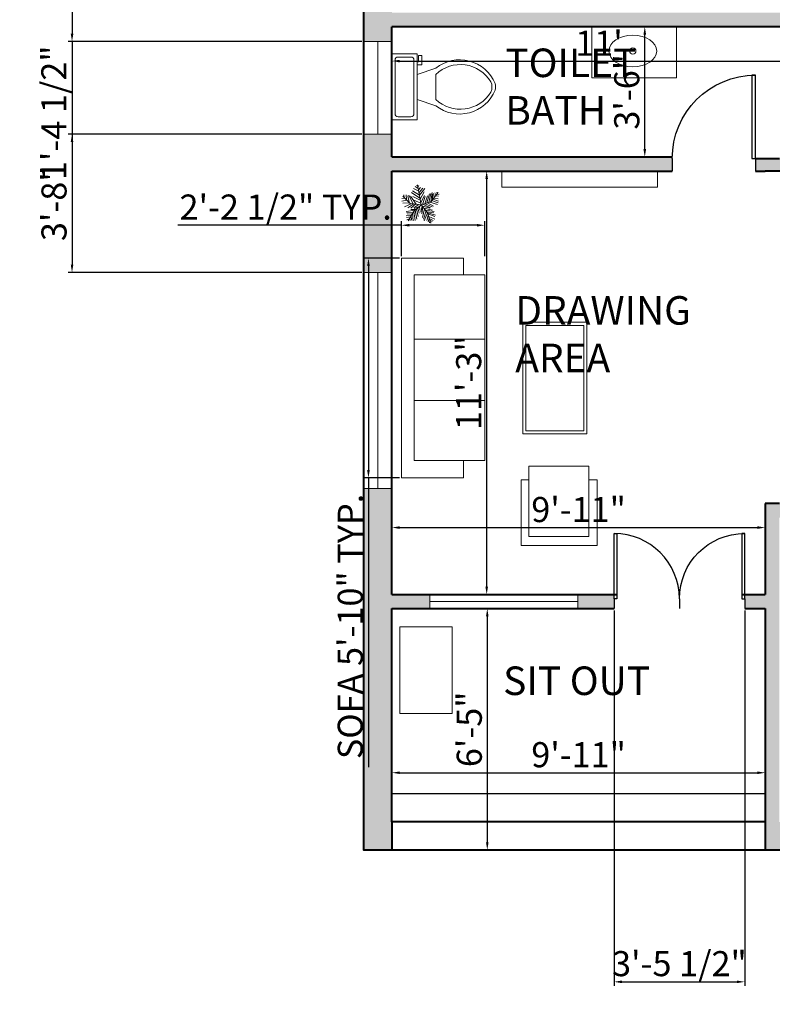
# Model space of a CAD drawing. Units: inches. Extents: x 529 to 1442, y 1029 to 1677.
# Tile 1 of 7: x 529 to 769, y 1098 to 1412. Entities that reach past the tile are written whole.
import ezdxf

# ---------------------------------------------------------------- set-up
doc = ezdxf.new("R2010")
doc.units = ezdxf.units.IN
for name, color, linetype, lineweight in [('A-ANNO-DIMS', 2, 'Continuous', 18), ('A-AREA-IDEN', 7, 'Continuous', 25), ('A-DOOR', 4, 'Continuous', 25), ('A-FLOR-FIXT', 9, 'Continuous', 18), ('A-FLOR-STRS', 7, 'Continuous', 25), ('A-FURN', 8, 'Continuous', 18), ('A-WALL-PATT', 252, 'Continuous', 13), ('tree', 70, 'Continuous', 13), ('wall', 7, 'Continuous', 40), ('window', 52, 'Continuous', 18)]:
    doc.layers.add(name, color=color, linetype=linetype, lineweight=lineweight)
doc.styles.get("Standard").update_dxf_attribs({"font": 'arial.ttf'})
doc.dimstyles.new('ISO-25', dxfattribs={"dimtxt": 8, "dimasz": 2.5, "dimexe": 1.25, "dimexo": 0.625, "dimtad": 1, "dimdec": 0, "dimlunit": 4, "dimtxsty": 'Standard', "dimcen": 2.5, "dimadec": 0, "dimazin": 0, "dimtfac": 1, "dimtdec": 0, "dimtmove": 0, "dimatfit": 3, "dimfxl": 1, "dimarcsym": 0})

# ---------------------------------------------------------------- blocks, each defined once
blk = doc.blocks.new('*U2')
for p, q in [((0, 0), (0, -6)), ((40, 0), (40, -6))]:
    blk.add_line(p, q)
blk.add_lwpolyline([(0, 0), (0, 40), (1.75, 40), (1.75, 0)], close=True)
blk.add_arc((0, 0), 40, 0, 90)
blk = doc.blocks.new('*U4')
for p, q in [((9.5, -6), (9.5, -2)), ((-10, -8.5), (-8, -8.5)), ((-10, -9.5), (-10, -8.5)), ((-8, -8.5), (-8, -8)), ((-7, -8), (-7, -9.5)), ((-4, -8), (-6, -14)), ((4, -8), (6, -14)), ((-7, -9.5), (-10, -9.5)), ((4, -14), (-4, -14))]:
    blk.add_line(p, q)
blk.add_lwpolyline([(10.5, -8), (10.5, 0), (-10.5, 0), (-10.5, -8)], close=True)
for points in [[(-9.5, -2), (-9.5, -6)], [(8.5, -1), (-8.5, -1)], [(-8.5, -7), (8.5, -7)]]:
    blk.add_lwpolyline(points)
for centre, radius, start, end in [((-8.62, -1.88), 0.884, 81.8699, 188.1301), ((8.62, -1.88), 0.884, 351.8699, 98.1301), ((-8.62, -6.12), 0.884, 171.8699, 278.1301), ((8.62, -6.12), 0.884, 261.8699, 8.1301), ((3.52, -21.58), 12.17, 141.4691, 247.9714), ((4.2, -21.82), 11.33, 136.3677, 238.9468), ((-3.52, -21.58), 12.17, 292.0284, 38.5307), ((-4.2, -21.82), 11.33, 301.053, 43.6321), ((0, -27.88), 4, 245.7318, 294.2682), ((0, -29), 4, 254.8605, 285.1395)]:
    blk.add_arc(centre, radius, start, end)
blk = doc.blocks.new('*U12')
for p, q in [((0, 0), (-10.5, 57)), ((-48.585, 21.131), (-49.309, 29.026)), ((-43.513, 28.561), (-42.427, 15.558)), ((-3.665, 19.273), (-27.574, 35.527)), ((-5.114, 28.097), (-24.676, 40.636)), ((-7.288, 39.707), (-21.778, 46.673)), ((-8.737, 47.138), (-17.069, 52.711)), ((-10.186, 53.64), (-13.084, 55.962)), ((-9.099, 51.782), (-6.563, 55.962)), ((-7.65, 43.423), (-2.578, 49.46)), ((-5.839, 35.992), (4.667, 48.067)), ((-5.114, 27.632), (10.463, 46.673)), ((-2.941, 16.486), (8.652, 37.85)), ((16.259, 5.805), (23.142, 31.348)), ((22.055, 7.198), (27.489, 32.277)), ((27, 9), (48, 36)), ((27.127, 9.056), (31.112, 35.992)), ((31.836, 30.883), (32.561, 16.486)), ((35.096, 32.741), (37.27, 22.524)), ((38.719, 34.134), (41.979, 28.561)), ((43.791, 29.954), (51.036, 30.883)), ((44.153, 36.456), (45.239, 32.741)), ((-47.498, 19.737), (-55.83, 18.344)), ((-40.615, 13.7), (-55.105, 10.913)), ((-31.5, 4.5), (-52.5, 25.5)), ((-33.37, 6.269), (-52.207, 5.34)), ((-28.299, 3.483), (-47.86, -5.805)), ((-38.442, 26.239), (-34.819, 7.663)), ((-21.416, 3.018), (-38.079, -8.128)), ((-35.544, 28.097), (-24.314, 3.947)), ((0, 0), (-31.5, 4.5)), ((-14.533, 2.09), (-30.834, 25.31)), ((-15.982, 2.09), (-30.11, -9.521)), ((-24.314, 23.917), (-2.941, 13.7)), ((0, 0), (-22.5, -19.5)), ((-6.563, 1.161), (-21.416, -8.128)), ((-20.691, 13.7), (-1.129, 4.876)), ((-1.129, 6.734), (9.014, 26.704)), ((0, 0), (27, 9)), ((0, 0), (18, -22.5)), ((3.942, 1.625), (11.187, 24.381)), ((6.478, 1.625), (26.04, -8.592)), ((10.101, 3.483), (17.708, 26.239)), ((11.187, 3.483), (30.749, -5.805)), ((18.07, 5.805), (35.096, -3.483)), ((24.229, 7.663), (46.688, 1.625)), ((29.662, 12.307), (48.137, 6.269)), ((33.285, 16.486), (48.862, 10.913)), ((36.183, 19.737), (48.137, 17.88)), ((40.53, 25.775), (48.862, 24.846)), ((-17.431, -15.094), (-42.789, -18.809)), ((-24.314, -21.596), (-42.427, -22.06)), ((-26.849, -26.24), (-40.253, -25.775)), ((-22.5, -19.5), (-37.5, -45)), ((-15.257, -12.772), (-30.11, -12.772)), ((-25.038, -23.918), (-22.865, -45.281)), ((-20.691, -18.345), (-17.793, -44.352)), ((-6.563, -5.805), (-19.967, -9.985)), ((-17.069, -15.094), (-12.721, -40.172)), ((-13.446, -11.378), (-8.737, -32.741)), ((-9.461, -8.592), (-6.201, -23.453)), ((-4.752, -3.483), (-3.665, -14.629)), ((2.493, -3.019), (-1.491, -20.202)), ((1.769, -2.555), (24.229, -9.521)), ((5.029, -6.27), (2.131, -25.775)), ((9.014, -11.378), (3.58, -35.992)), ((14.085, -16.951), (6.478, -40.172)), ((7.565, -9.056), (32.198, -14.629)), ((18.07, -22.524), (8.289, -45.745)), ((12.274, -15.094), (36.907, -18.809)), ((16.259, -19.738), (36.183, -22.989)), ((18, -22.5), (27, -52.5)), ((18.433, -22.524), (40.53, -29.026)), ((19.157, -25.311), (38.719, -33.206)), ((-28.299, -29.026), (-42.789, -31.348)), ((-30.834, -34.135), (-42.427, -35.528)), ((-34.457, -39.708), (-40.978, -42.494)), ((-32.646, -36.921), (-31.921, -44.352)), ((-29.023, -30.884), (-27.936, -43.887)), ((20.244, -30.419), (15.897, -44.816)), ((22.78, -37.85), (19.519, -48.532)), ((21.331, -32.741), (39.081, -40.636)), ((22.78, -38.314), (34.372, -44.816)), ((24.591, -45.745), (23.142, -50.854)), ((24.591, -43.423), (30.749, -47.603)), ((26.764, -49.925), (28.213, -50.854))]:
    blk.add_line(p, q)
blk = doc.blocks.new('*D39')
at = {"layer": 'A-ANNO-DIMS', "color": 0, "lineweight": -2, "transparency": 16777216}
for p, q in [((647.38, 1165.44), (647.38, 1172.73)), ((649.88, 1171.48), (763.88, 1171.48)), ((766.38, 1165.44), (766.38, 1172.73))]:
    blk.add_line(p, q, dxfattribs=at)
at = {"layer": 'A-ANNO-DIMS', "color": 0, "lineweight": 100, "transparency": 16777216}
for points in [[(649.88, 1171.89), (649.88, 1171.06), (647.38, 1171.48)], [(763.88, 1171.89), (763.88, 1171.06), (766.38, 1171.48)]]:
    blk.add_solid(points, dxfattribs=at)
at = {"layer": 'Defpoints', "color": 0, "lineweight": 100, "transparency": 16777216}
for p in [(766.38, 1171.48), (647.38, 1164.81), (766.38, 1164.81)]:
    blk.add_point(p, dxfattribs=at)
at = {"layer": 'A-ANNO-DIMS', "color": 0, "transparency": 16777216, "insert": (706.88, 1176.19), "char_height": 8, "attachment_point": 5}
blk.add_mtext('9\'-11"', dxfattribs=at)
blk = doc.blocks.new('*D40')
at = {"layer": 'A-ANNO-DIMS', "color": 0, "lineweight": -2, "transparency": 16777216}
for p, q in [((648.01, 1223.81), (679.01, 1223.81)), ((677.76, 1221.31), (677.76, 1149.31)), ((648.01, 1146.81), (679.01, 1146.81))]:
    blk.add_line(p, q, dxfattribs=at)
at = {"layer": 'A-ANNO-DIMS', "color": 0, "lineweight": 100, "transparency": 16777216}
for points in [[(677.35, 1221.31), (678.18, 1221.31), (677.76, 1223.81)], [(677.35, 1149.31), (678.18, 1149.31), (677.76, 1146.81)]]:
    blk.add_solid(points, dxfattribs=at)
at = {"layer": 'Defpoints', "color": 0, "lineweight": 100, "transparency": 16777216}
for p in [(647.38, 1223.81), (647.38, 1146.81), (677.76, 1146.81)]:
    blk.add_point(p, dxfattribs=at)
at = {"layer": 'A-ANNO-DIMS', "color": 0, "transparency": 16777216, "insert": (673.06, 1185.31), "char_height": 8, "attachment_point": 5, "rotation": 90}
blk.add_mtext('6\'-5"', dxfattribs=at)
blk = doc.blocks.new('*D41')
at = {"layer": 'A-ANNO-DIMS', "color": 0, "lineweight": -2, "transparency": 16777216}
for p, q in [((648.01, 1363.31), (678.82, 1363.31)), ((677.57, 1230.81), (677.57, 1360.81)), ((648.01, 1228.31), (678.82, 1228.31))]:
    blk.add_line(p, q, dxfattribs=at)
at = {"layer": 'A-ANNO-DIMS', "color": 0, "lineweight": 100, "transparency": 16777216}
for points in [[(677.16, 1360.81), (677.99, 1360.81), (677.57, 1363.31)], [(677.16, 1230.81), (677.99, 1230.81), (677.57, 1228.31)]]:
    blk.add_solid(points, dxfattribs=at)
at = {"layer": 'Defpoints', "color": 0, "lineweight": 100, "transparency": 16777216}
for p in [(647.38, 1363.31), (677.57, 1363.31), (647.38, 1228.31)]:
    blk.add_point(p, dxfattribs=at)
at = {"layer": 'A-ANNO-DIMS', "color": 0, "transparency": 16777216, "insert": (672.86, 1295.81), "char_height": 8, "attachment_point": 5, "rotation": 90}
blk.add_mtext('11\'-3"', dxfattribs=at)
blk = doc.blocks.new('*D42')
at = {"layer": 'A-ANNO-DIMS', "color": 0, "lineweight": -2, "transparency": 16777216}
for p, q in [((647.38, 1228.94), (647.38, 1250.89)), ((649.88, 1249.64), (763.88, 1249.64)), ((766.38, 1228.94), (766.38, 1250.89))]:
    blk.add_line(p, q, dxfattribs=at)
at = {"layer": 'A-ANNO-DIMS', "color": 0, "lineweight": 100, "transparency": 16777216}
for points in [[(649.88, 1250.06), (649.88, 1249.22), (647.38, 1249.64)], [(763.88, 1250.06), (763.88, 1249.22), (766.38, 1249.64)]]:
    blk.add_solid(points, dxfattribs=at)
at = {"layer": 'Defpoints', "color": 0, "lineweight": 100, "transparency": 16777216}
for p in [(766.38, 1249.64), (647.38, 1228.31), (766.38, 1228.31)]:
    blk.add_point(p, dxfattribs=at)
at = {"layer": 'A-ANNO-DIMS', "color": 0, "transparency": 16777216, "insert": (706.88, 1254.35), "char_height": 8, "attachment_point": 5}
blk.add_mtext('9\'-11"', dxfattribs=at)
blk = doc.blocks.new('*D45')
at = {"layer": 'A-ANNO-DIMS', "color": 0, "lineweight": -2, "transparency": 16777216}
for p, q in [((647.38, 1408.69), (647.38, 1397.12)), ((779.38, 1408.69), (779.38, 1397.12)), ((649.88, 1398.37), (776.88, 1398.37))]:
    blk.add_line(p, q, dxfattribs=at)
at = {"layer": 'A-ANNO-DIMS', "color": 0, "lineweight": 100, "transparency": 16777216}
for points in [[(649.88, 1398.78), (649.88, 1397.95), (647.38, 1398.37)], [(776.88, 1398.78), (776.88, 1397.95), (779.38, 1398.37)]]:
    blk.add_solid(points, dxfattribs=at)
at = {"layer": 'Defpoints', "color": 0, "lineweight": 100, "transparency": 16777216}
for p in [(647.38, 1409.31), (779.38, 1409.31), (779.38, 1398.37)]:
    blk.add_point(p, dxfattribs=at)
at = {"layer": 'A-ANNO-DIMS', "color": 0, "transparency": 16777216, "insert": (713.38, 1403.01), "char_height": 8, "attachment_point": 5}
blk.add_mtext("11'", dxfattribs=at)
blk = doc.blocks.new('*D46')
at = {"layer": 'A-ANNO-DIMS', "color": 0, "lineweight": -2, "transparency": 16777216}
for p, q in [((648.01, 1409.31), (729.23, 1409.31)), ((727.98, 1370.31), (727.98, 1406.81)), ((648.01, 1367.81), (729.23, 1367.81))]:
    blk.add_line(p, q, dxfattribs=at)
at = {"layer": 'A-ANNO-DIMS', "color": 0, "lineweight": 100, "transparency": 16777216}
for points in [[(727.56, 1406.81), (728.4, 1406.81), (727.98, 1409.31)], [(727.56, 1370.31), (728.4, 1370.31), (727.98, 1367.81)]]:
    blk.add_solid(points, dxfattribs=at)
at = {"layer": 'Defpoints', "color": 0, "lineweight": 100, "transparency": 16777216}
for p in [(647.38, 1409.31), (727.98, 1409.31), (647.38, 1367.81)]:
    blk.add_point(p, dxfattribs=at)
at = {"layer": 'A-ANNO-DIMS', "color": 0, "transparency": 16777216, "insert": (723.27, 1388.56), "char_height": 8, "attachment_point": 5, "rotation": 90}
blk.add_mtext('3\'-6"', dxfattribs=at)
blk = doc.blocks.new('WIN-LARGE-PLAN')
blk.add_line((0, 4.5), (68.85, 4.5))
blk.add_lwpolyline([(0, 9), (68.85, 9), (68.85, 0), (0, 0)], close=True)
blk = doc.blocks.new('WIN-VENT-PLAN')
blk.add_line((4.5, 0), (4.5, 29.5))
blk.add_lwpolyline([(0, 29.5), (9, 29.5), (9, 0), (0, 0)], close=True)
blk = doc.blocks.new('SOFA-THREE-SEAT')
for p, q in [((6.71, 64.51), (6.71, 70.05)), ((6.71, 70.05), (26.55, 70.05)), ((26.55, 70.05), (26.55, 0)), ((0, 45.39), (22.47, 45.39)), ((0, 25.77), (22.47, 25.77)), ((6.71, 0), (6.71, 5.33)), ((26.55, 0), (6.71, 0))]:
    blk.add_line(p, q)
for points in [[(22.47, 64.51), (0, 64.51), (0, 5.33), (22.47, 5.33)], [(0, 45.39), (22.47, 45.39), (22.47, 64.51), (0, 64.51)]]:
    blk.add_lwpolyline(points, close=True)
blk = doc.blocks.new('LOUNGE-CHAIR')
for p, q in [((0, 4.37), (0, 25.3)), ((0, 25.3), (24.27, 25.3)), ((24.27, 25.3), (24.27, 4.37)), ((2.68, 4.37), (0, 4.37)), ((2.68, 4.37), (2.68, 4.37)), ((24.27, 4.37), (21.8, 4.37))]:
    blk.add_line(p, q)
blk.add_lwpolyline([(2.68, 22.46), (2.68, 0), (21.8, 0), (21.8, 22.46)], close=True)
blk = doc.blocks.new('COFFEE-TABLE')
for points in [[(0, 35.56), (20.45, 35.56), (20.45, 0), (0, 0)], [(1, 34.56), (19.45, 34.56), (19.45, 1), (1, 1)]]:
    blk.add_lwpolyline(points, close=True)
blk = doc.blocks.new('WASHBASIN')
blk.add_lwpolyline([(0, 16.29), (27.02, 16.29), (27.02, 0), (0, 0)], close=True)
blk.add_circle((13.05, 8.54), 0.991)
blk.add_ellipse((13.05, 8.54), major_axis=(7.63, 0), ratio=0.659433)
blk = doc.blocks.new('*D89')
at = {"layer": 'A-ANNO-DIMS', "color": 0, "lineweight": -2, "transparency": 16777216}
for p, q in [((649.76, 1335.52), (638.63, 1335.52)), ((639.88, 1333.02), (639.88, 1267.98)), ((649.76, 1265.48), (638.63, 1265.48)), ((639.88, 1265.48), (639.88, 1173.25))]:
    blk.add_line(p, q, dxfattribs=at)
at = {"layer": 'A-ANNO-DIMS', "color": 0, "lineweight": 100, "transparency": 16777216}
for points in [[(639.46, 1333.02), (640.3, 1333.02), (639.88, 1335.52)], [(639.46, 1267.98), (640.3, 1267.98), (639.88, 1265.48)]]:
    blk.add_solid(points, dxfattribs=at)
at = {"layer": 'Defpoints', "color": 0, "lineweight": 100, "transparency": 16777216}
for p in [(650.39, 1335.52), (639.88, 1265.48), (650.39, 1265.48)]:
    blk.add_point(p, dxfattribs=at)
at = {"layer": 'A-ANNO-DIMS', "color": 0, "transparency": 16777216, "insert": (635.12, 1218.11), "char_height": 8, "attachment_point": 5, "rotation": 90}
blk.add_mtext('SOFA 5\'-10" TYP.', dxfattribs=at)
blk = doc.blocks.new('*D90')
at = {"layer": 'A-ANNO-DIMS', "color": 0, "lineweight": -2, "transparency": 16777216}
for p, q in [((650.39, 1336.15), (650.39, 1347.28)), ((676.94, 1336.15), (676.94, 1347.28)), ((650.39, 1346.03), (579.1, 1346.03)), ((674.44, 1346.03), (652.89, 1346.03))]:
    blk.add_line(p, q, dxfattribs=at)
at = {"layer": 'A-ANNO-DIMS', "color": 0, "lineweight": 100, "transparency": 16777216}
for points in [[(652.89, 1346.45), (652.89, 1345.61), (650.39, 1346.03)], [(674.44, 1346.45), (674.44, 1345.61), (676.94, 1346.03)]]:
    blk.add_solid(points, dxfattribs=at)
at = {"layer": 'Defpoints', "color": 0, "lineweight": 100, "transparency": 16777216}
for p in [(650.39, 1346.03), (650.39, 1335.52), (676.94, 1335.52)]:
    blk.add_point(p, dxfattribs=at)
at = {"layer": 'A-ANNO-DIMS', "color": 0, "transparency": 16777216, "insert": (613.49, 1350.79), "char_height": 8, "attachment_point": 5}
blk.add_mtext('2\'-2 1/2" TYP.', dxfattribs=at)
blk = doc.blocks.new('*D106')
at = {"layer": 'A-ANNO-DIMS', "color": 0, "lineweight": -2, "transparency": 16777216}
for p, q in [((637.76, 1420.96), (544.13, 1420.96)), ((545.38, 1418.46), (545.38, 1407.08)), ((637.76, 1404.58), (544.13, 1404.58)), ((545.38, 1404.58), (545.38, 1361.68))]:
    blk.add_line(p, q, dxfattribs=at)
at = {"layer": 'A-ANNO-DIMS', "color": 0, "lineweight": 100, "transparency": 16777216}
for points in [[(544.97, 1418.46), (545.8, 1418.46), (545.38, 1420.96)], [(544.97, 1407.08), (545.8, 1407.08), (545.38, 1404.58)]]:
    blk.add_solid(points, dxfattribs=at)
at = {"layer": 'Defpoints', "color": 0, "lineweight": 100, "transparency": 16777216}
for p in [(638.38, 1420.96), (545.38, 1404.58), (638.38, 1404.58)]:
    blk.add_point(p, dxfattribs=at)
at = {"layer": 'A-ANNO-DIMS', "color": 0, "transparency": 16777216, "insert": (540.62, 1381.88), "char_height": 8, "attachment_point": 5, "rotation": 90}
blk.add_mtext('1\'-4 1/2"', dxfattribs=at)
blk = doc.blocks.new('*D107')
at = {"layer": 'A-ANNO-DIMS', "color": 0, "lineweight": -2, "transparency": 16777216}
for p, q in [((637.76, 1375.08), (544.13, 1375.08)), ((545.38, 1372.58), (545.38, 1333.47)), ((637.76, 1330.97), (544.13, 1330.97))]:
    blk.add_line(p, q, dxfattribs=at)
at = {"layer": 'A-ANNO-DIMS', "color": 0, "lineweight": 100, "transparency": 16777216}
for points in [[(544.97, 1372.58), (545.8, 1372.58), (545.38, 1375.08)], [(544.97, 1333.47), (545.8, 1333.47), (545.38, 1330.97)]]:
    blk.add_solid(points, dxfattribs=at)
at = {"layer": 'Defpoints', "color": 0, "lineweight": 100, "transparency": 16777216}
for p in [(638.38, 1375.08), (545.38, 1330.97), (638.38, 1330.97)]:
    blk.add_point(p, dxfattribs=at)
at = {"layer": 'A-ANNO-DIMS', "color": 0, "transparency": 16777216, "insert": (540.67, 1353.03), "char_height": 8, "attachment_point": 5, "rotation": 90}
blk.add_mtext('3\'-8"', dxfattribs=at)
blk = doc.blocks.new('*D115')
at = {"layer": 'A-ANNO-DIMS', "color": 0, "lineweight": -2, "transparency": 16777216}
for p, q in [((718.19, 1223.19), (718.19, 1103.56)), ((759.84, 1223.19), (759.84, 1103.56)), ((720.69, 1104.81), (757.34, 1104.81))]:
    blk.add_line(p, q, dxfattribs=at)
at = {"layer": 'A-ANNO-DIMS', "color": 0, "lineweight": 100, "transparency": 16777216}
for points in [[(720.69, 1105.23), (720.69, 1104.4), (718.19, 1104.81)], [(757.34, 1105.23), (757.34, 1104.4), (759.84, 1104.81)]]:
    blk.add_solid(points, dxfattribs=at)
at = {"layer": 'Defpoints', "color": 0, "lineweight": 100, "transparency": 16777216}
for p in [(718.19, 1223.81), (759.84, 1223.81), (759.84, 1104.81)]:
    blk.add_point(p, dxfattribs=at)
at = {"layer": 'A-ANNO-DIMS', "color": 0, "transparency": 16777216, "insert": (739.02, 1109.58), "char_height": 8, "attachment_point": 5}
blk.add_mtext('3\'-5 1/2"', dxfattribs=at)

msp = doc.modelspace()

# ---------------------------------------------------------------- hatches: boundary and pattern name
at = {"layer": 'A-WALL-PATT'}
h = msp.add_hatch(color=256, dxfattribs=at)
h.dxf.hatch_style = 1
h.paths.add_polyline_path([(678.78, 1566.81), (638.38, 1566.81), (638.38, 1489.81), (647.38, 1489.81), (647.38, 1557.81), (678.78, 1557.81)])
h.paths.add_polyline_path([(805.14, 1566.81), (747.64, 1566.81), (747.64, 1557.81), (779.38, 1557.81), (805.14, 1557.81)])
h.paths.add_polyline_path([(890.86, 1566.81), (836.43, 1566.81), (836.43, 1557.81), (854.88, 1557.81), (890.86, 1557.81)])
h.paths.add_polyline_path([(783.88, 1557.81), (779.38, 1557.81), (779.38, 1505.45), (783.88, 1505.45)])
h.paths.add_polyline_path([(783.88, 1472.6), (779.38, 1472.6), (779.38, 1456.82), (783.88, 1456.82)])
h.paths.add_polyline_path([(859.38, 1557.81), (854.88, 1557.81), (854.88, 1467.81), (783.88, 1467.81), (783.88, 1463.31), (859.38, 1463.31)])
h.paths.add_polyline_path([(859.38, 1463.31), (854.88, 1463.31), (854.88, 1409.31), (864.07, 1409.31), (864.07, 1413.81), (859.38, 1413.81)])
h.paths.add_polyline_path([(647.38, 1420.96), (638.38, 1420.96), (638.38, 1404.58), (647.38, 1404.58)])
h.paths.add_polyline_path([(779.38, 1413.81), (647.38, 1413.81), (647.38, 1409.31), (779.38, 1409.31)])
h.paths.add_polyline_path([(647.38, 1363.31), (647.38, 1375.08), (638.38, 1375.08), (638.38, 1330.97), (647.38, 1330.97)])
h.paths.add_polyline_path([(736.73, 1367.3, -0.004844), (736.74, 1367.81), (647.38, 1367.81), (647.38, 1363.31), (736.73, 1363.31)])
h.paths.add_polyline_path([(783.88, 1409.31), (779.38, 1409.31), (779.38, 1367.36), (770.88, 1367.36), (770.88, 1363.31), (783.88, 1363.31)])
h.paths.add_polyline_path([(770.88, 1367.36), (763.3, 1367.36), (763.3, 1367.3), (763.3, 1363.31), (766.38, 1363.31), (770.88, 1363.31)])
h.paths.add_polyline_path([(783.88, 1416.82), (779.38, 1416.82), (779.38, 1413.81), (779.38, 1409.31), (783.88, 1409.31)])
h.paths.add_polyline_path([(647.38, 1223.81), (647.38, 1262.11), (638.38, 1262.11), (638.38, 1146.81), (647.38, 1146.81), (647.38, 1155.81)])
h.paths.add_polyline_path([(659.49, 1228.31), (647.38, 1228.31), (647.38, 1223.81), (659.49, 1223.81)])
h.paths.add_polyline_path([(718.19, 1226.94), (718.19, 1228.31), (706.68, 1228.31), (706.68, 1223.81), (718.19, 1223.81)])
h.paths.add_polyline_path([(770.88, 1252.81), (786.93, 1252.81), (786.93, 1257.31), (770.88, 1257.31), (766.38, 1257.31), (766.38, 1228.31), (759.84, 1228.31), (759.84, 1226.94), (759.84, 1223.81), (766.38, 1223.81), (766.38, 1155.81), (770.88, 1155.81), (770.88, 1179.81)])
h.paths.add_polyline_path([(794.05, 1155.81), (766.38, 1155.81), (766.38, 1146.81), (794.05, 1146.81)])
h.paths.add_polyline_path([(859.38, 1155.81), (825.34, 1155.81), (825.34, 1146.81), (859.38, 1146.81)])

# ---------------------------------------------------------------- linework, layer by layer
at = {"layer": 'A-FLOR-STRS'}
for p, q in [((647.21, 1164.81), (766.21, 1164.81)), ((647.38, 1155.81), (766.38, 1155.81))]:
    msp.add_line(p, q, dxfattribs=at)
at = {"layer": 'A-FURN'}
for points in [[(682.45, 1363.31), (731.98, 1363.31), (731.98, 1358.19), (682.45, 1358.19)], [(649.86, 1218.01), (666.59, 1218.01), (666.59, 1190.34), (649.86, 1190.34)]]:
    msp.add_lwpolyline(points, close=True, dxfattribs=at)
at = {"layer": 'wall'}
for p, q in [((638.38, 1146.81), (638.38, 1566.81)), ((779.38, 1409.31), (647.38, 1409.31)), ((647.38, 1367.81), (736.74, 1367.81)), ((763.3, 1367.36), (770.88, 1367.36)), ((647.38, 1228.31), (647.38, 1363.31)), ((647.38, 1363.31), (736.73, 1363.31)), ((763.3, 1363.31), (766.38, 1363.31)), ((783.88, 1363.31), (766.38, 1363.31)), ((766.38, 1257.31), (766.38, 1228.31)), ((770.88, 1257.31), (766.38, 1257.31)), ((647.38, 1228.31), (719.11, 1228.31)), ((738.97, 1228.31), (739.06, 1228.31)), ((758.93, 1228.31), (766.38, 1228.31)), ((647.38, 1155.81), (647.38, 1223.81)), ((647.38, 1223.81), (718.19, 1223.81)), ((759.84, 1223.81), (766.38, 1223.81)), ((766.38, 1223.81), (766.38, 1155.81)), ((647.38, 1155.81), (647.38, 1146.81)), ((766.38, 1155.81), (766.38, 1146.81)), ((859.38, 1146.81), (638.38, 1146.81))]:
    msp.add_line(p, q, dxfattribs=at)
for points in [[(859.38, 1146.81), (638.38, 1146.81), (638.38, 1566.81), (1358.38, 1566.81), (1358.38, 1146.81), (1132.38, 1146.81)], [(647.38, 1367.81), (647.38, 1409.31)], [(647.38, 1228.31), (647.38, 1363.31)], [(766.38, 1155.81), (647.38, 1155.81), (647.38, 1223.81)]]:
    msp.add_lwpolyline(points, dxfattribs=at)
at = {"layer": 'window'}
msp.add_line((659.49, 1226.06), (706.68, 1226.06), dxfattribs=at)
msp.add_lwpolyline([(659.49, 1228.31), (706.68, 1228.31), (706.68, 1223.81), (659.49, 1223.81)], close=True, dxfattribs=at)

# ---------------------------------------------------------------- block references
at = {"layer": 'A-DOOR'}
for p, xscale, yscale, zscale in [((763.3, 1367.3), -0.6642090761901391, 0.6642090761901391, 0.6642090761901391), ((718.19, 1226.94), 0.5205824161454354, 0.5205824161454354, 0.5205824161454354), ((759.84, 1226.94), -0.5205824161454354, 0.5205824161454354, 0.5205824161454354)]:
    msp.add_blockref('*U2', p, dxfattribs=dict(at, xscale=xscale, yscale=yscale, zscale=zscale))
at = {"layer": 'A-FLOR-FIXT'}
msp.add_blockref('WASHBASIN', (711.11, 1393.02), dxfattribs=at)
at = {"layer": 'A-FLOR-FIXT', "xscale": -1, "rotation": 90}
msp.add_blockref('*U4', (647.38, 1390.14), dxfattribs=at)
at = {"layer": 'A-FURN', "rotation": 180}
for name, p in [('SOFA-THREE-SEAT', (676.94, 1335.52)), ('COFFEE-TABLE', (709.53, 1315.08)), ('LOUNGE-CHAIR', (712.85, 1269.26))]:
    msp.add_blockref(name, p, dxfattribs=at)
at = {"layer": 'tree', "xscale": 0.1116431773080361, "yscale": 0.1116431773080361, "zscale": 0.1116431773080361}
msp.add_blockref('*U12', (656.71, 1352.5), dxfattribs=at)
at = {"layer": 'window'}
msp.add_blockref('WIN-VENT-PLAN', (638.38, 1375.08), dxfattribs=at)
at = {"layer": 'window', "rotation": 269.9999999999996}
msp.add_blockref('WIN-LARGE-PLAN', (638.38, 1330.97), dxfattribs=at)

# ---------------------------------------------------------------- texts
at = {"layer": 'A-AREA-IDEN', "char_height": 9.098, "attachment_point": 1}
for s, insert in [('TOILET\\PBATH', (683.51, 1402.36)), ('DRAWING\\PAREA', (686.68, 1323.43)), ('SIT OUT', (682.82, 1205.35))]:
    msp.add_mtext_dynamic_manual_height_columns(s, width=307.5887, gutter_width=45.49, heights=[0], dxfattribs=dict(at, insert=insert))

# ---------------------------------------------------------------- dimensions: what is measured, and where the dimension line sits
at = {"layer": 'A-ANNO-DIMS'}
for base, p1, p2, override, picture, middle in [((545.38, 1404.58), (638.38, 1420.96), (638.38, 1404.58), {"dimdec": 1, "dimlfac": 1, "dimrnd": 0, "dimzin": 1, "dimdsep": 46, "dimlunit": 4, "dimfrac": 2}, '*D106', (540.62, 1381.88)), ((545.38, 1330.97), (638.38, 1375.08), (638.38, 1330.97), {"dimdec": 1, "dimlfac": 1, "dimrnd": 0, "dimzin": 1, "dimdsep": 46, "dimlunit": 4, "dimfrac": 2}, '*D107', (540.67, 1353.03)), ((677.57, 1363.31), (647.38, 1228.31), (647.38, 1363.31), {"dimclrd": 0, "dimclre": 0, "dimclrt": 0}, '*D41', (672.86, 1295.81)), ((677.76, 1146.81), (647.38, 1223.81), (647.38, 1146.81), {"dimclrd": 0, "dimclre": 0, "dimclrt": 0}, '*D40', (673.06, 1185.31))]:
    dim = msp.add_linear_dim(base=base, p1=p1, p2=p2, angle=90, dimstyle='ISO-25', override=override, dxfattribs=at)
    dim.commit()
    dim.dimension.update_dxf_attribs({"geometry": picture, "text_midpoint": middle})
for base, p1, p2, override, picture, middle in [((779.38, 1398.37), (647.38, 1409.31), (779.38, 1409.31), {"dimclrd": 0, "dimclre": 0, "dimclrt": 0}, '*D45', (713.38, 1403.01)), ((766.38, 1249.64), (647.38, 1228.31), (766.38, 1228.31), {"dimclrd": 0, "dimclre": 0, "dimclrt": 0}, '*D42', (706.88, 1254.35)), ((759.841, 1104.8124), (718.1944, 1223.8124), (759.841, 1223.8124), {"dimdec": 1, "dimlfac": 1, "dimrnd": 0, "dimzin": 1, "dimdsep": 46, "dimlunit": 4, "dimfrac": 2}, '*D115', (739.0177, 1109.5766)), ((766.38, 1171.48), (647.38, 1164.81), (766.38, 1164.81), {"dimclrd": 0, "dimclre": 0, "dimclrt": 0}, '*D39', (706.88, 1176.19))]:
    dim = msp.add_linear_dim(base=base, p1=p1, p2=p2, dimstyle='ISO-25', override=override, dxfattribs=at)
    dim.commit()
    dim.dimension.update_dxf_attribs({"geometry": picture, "text_midpoint": middle})
dim = msp.add_aligned_dim(p1=(647.38418487, 1367.81239608), p2=(647.38418487, 1409.31239608), distance=-80.59735559, dimstyle='ISO-25', override={"dimclrd": 0, "dimclre": 0, "dimclrt": 0}, dxfattribs=at)
dim.commit()
dim.dimension.update_dxf_attribs({"geometry": '*D46', "text_midpoint": (723.26922804, 1388.56239608)})
for base, p1, p2, angle, text, picture, middle in [((650.388, 1346.0285), (676.9374, 1335.5216), (650.388, 1335.5216), 180, '<> TYP.', '*D90', (613.4922, 1350.79)), ((639.88, 1265.48), (650.39, 1335.52), (650.39, 1265.48), 270, 'SOFA <> TYP.', '*D89', (635.12, 1218.11))]:
    dim = msp.add_linear_dim(base=base, p1=p1, p2=p2, angle=angle, text=text, dimstyle='ISO-25', override={"dimdec": 1, "dimlfac": 1, "dimrnd": 0, "dimzin": 1, "dimdsep": 46, "dimlunit": 4, "dimfrac": 2}, dxfattribs=at)
    dim.commit()
    dim.dimension.update_dxf_attribs({"geometry": picture, "text_midpoint": middle})

doc.saveas('drawing.dxf')
